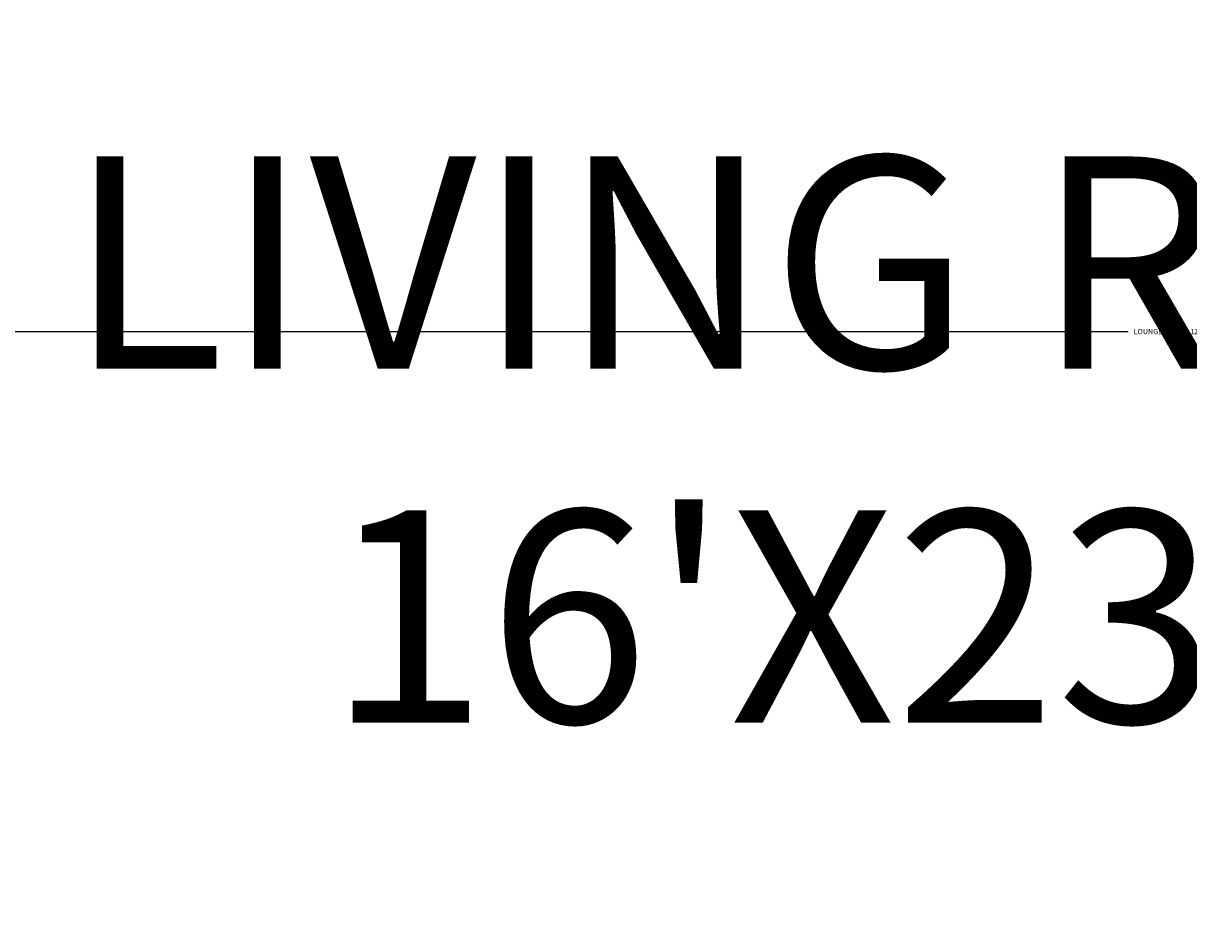
# Model space of a CAD drawing. Units: inches. Extents: x 182 to 1022, y -617 to 111.
# Tile 3 of 33: x 294 to 334, y -340 to -309. Entities that reach past the tile are written whole.
import ezdxf

# ---------------------------------------------------------------- set-up
doc = ezdxf.new("R2010")
doc.units = ezdxf.units.IN
doc.header["$MEASUREMENT"] = 0
doc.layers.add('A-ANNO-DIMS', color=2, linetype='Continuous', lineweight=18)
doc.layers.add('A-AREA-IDEN', color=8, linetype='Continuous', lineweight=18)
doc.styles.get("Standard").update_dxf_attribs({"font": 'arial.ttf'})
doc.dimstyles.get("Standard").update_dxf_attribs({"dimtxt": 0.18, "dimasz": 0.18, "dimexe": 0.18, "dimexo": 0.0625, "dimgap": 0.09, "dimtad": 0, "dimtih": 1, "dimtoh": 1, "dimdec": 1, "dimzin": 0, "dimdsep": 46, "dimlunit": 4, "dimtxsty": 'Standard', "dimcen": 0.09, "dimadec": 0, "dimazin": 0, "dimtfac": 1, "dimtdec": 1, "dimtofl": 0, "dimtmove": 0, "dimatfit": 3, "dimfxl": 1, "dimtolj": 1, "dimtzin": 0, "dimarcsym": 0})

# ---------------------------------------------------------------- blocks, each defined once
blk = doc.blocks.new('*D26')
at = {"layer": 'A-ANNO-DIMS', "color": 0, "lineweight": -2, "transparency": 16777216}
for p, q in [((257.848, -296.884), (257.848, -319.733)), ((409.388, -296.884), (409.388, -319.733)), ((258.028, -319.553), (331.642, -319.553)), ((409.208, -319.553), (335.594, -319.553))]:
    blk.add_line(p, q, dxfattribs=at)
at = {"layer": 'A-ANNO-DIMS', "color": 0, "transparency": 16777216}
for points in [[(258.028, -319.523), (258.028, -319.583), (257.848, -319.553)], [(409.208, -319.523), (409.208, -319.583), (409.388, -319.553)]]:
    blk.add_solid(points, dxfattribs=at)
at = {"layer": 'Defpoints', "color": 0, "transparency": 16777216}
for p in [(257.848, -296.822), (409.388, -296.822), (409.388, -319.553)]:
    blk.add_point(p, dxfattribs=at)
at = {"layer": 'A-ANNO-DIMS', "color": 0, "transparency": 16777216, "insert": (333.618, -319.553), "char_height": 0.18, "attachment_point": 5}
blk.add_mtext('\\A1;LOUNGE GROUP 12\'-7 1/2" TYP.', dxfattribs=at)
blk = doc.blocks.new('*D39')
at = {"layer": 'A-ANNO-DIMS', "color": 0, "lineweight": -2, "transparency": 16777216}
for p, q in [((238.398, -288.54), (1015.285, -288.54)), ((1015.105, -288.72), (1015.105, -346.775)), ((1015.105, -405.193), (1015.105, -347.138)), ((238.427, -405.373), (1015.285, -405.373))]:
    blk.add_line(p, q, dxfattribs=at)
at = {"layer": 'A-ANNO-DIMS', "color": 0, "transparency": 16777216}
for points in [[(1015.075, -288.72), (1015.135, -288.72), (1015.105, -288.54)], [(1015.075, -405.193), (1015.135, -405.193), (1015.105, -405.373)]]:
    blk.add_solid(points, dxfattribs=at)
at = {"layer": 'Defpoints', "color": 0, "transparency": 16777216}
for p in [(238.335, -288.54), (1015.105, -288.54), (238.364, -405.373)]:
    blk.add_point(p, dxfattribs=at)
at = {"layer": 'A-ANNO-DIMS', "color": 0, "transparency": 16777216, "insert": (1015.105, -346.956), "char_height": 0.18, "attachment_point": 5}
blk.add_mtext('\\A1;9\'-9"', dxfattribs=at)

msp = doc.modelspace()

# ---------------------------------------------------------------- texts
at = {"layer": 'A-AREA-IDEN', "insert": (286.446, -313.558), "char_height": 7.27028, "attachment_point": 1}
msp.add_mtext_dynamic_manual_height_columns('    LIVING ROOM\\P        16\'X23\'3"', width=90.78123, gutter_width=1.212, heights=[0], dxfattribs=at)

# ---------------------------------------------------------------- dimensions: what is measured, and where the dimension line sits
at = {"layer": 'A-ANNO-DIMS'}
dim = msp.add_linear_dim(base=(1015.105, -288.54), p1=(238.364, -405.373), p2=(238.335, -288.54), angle=90, dimstyle='Standard', override={"dimdec": 1, "dimlfac": 1, "dimrnd": 0, "dimzin": 1, "dimdsep": 46, "dimlunit": 4, "dimfrac": 2}, dxfattribs=at)
dim.commit()
dim.dimension.update_dxf_attribs({"geometry": '*D39', "text_midpoint": (1015.105, -346.956)})
dim = msp.add_linear_dim(base=(409.388, -319.553), p1=(257.848, -296.822), p2=(409.388, -296.822), text='LOUNGE GROUP <> TYP.', dimstyle='Standard', override={"dimdec": 1, "dimlfac": 1, "dimrnd": 0, "dimzin": 1, "dimdsep": 46, "dimlunit": 4, "dimfrac": 2}, dxfattribs=at)
dim.commit()
dim.dimension.update_dxf_attribs({"geometry": '*D26', "text_midpoint": (333.618, -319.553)})

doc.saveas('drawing.dxf')
